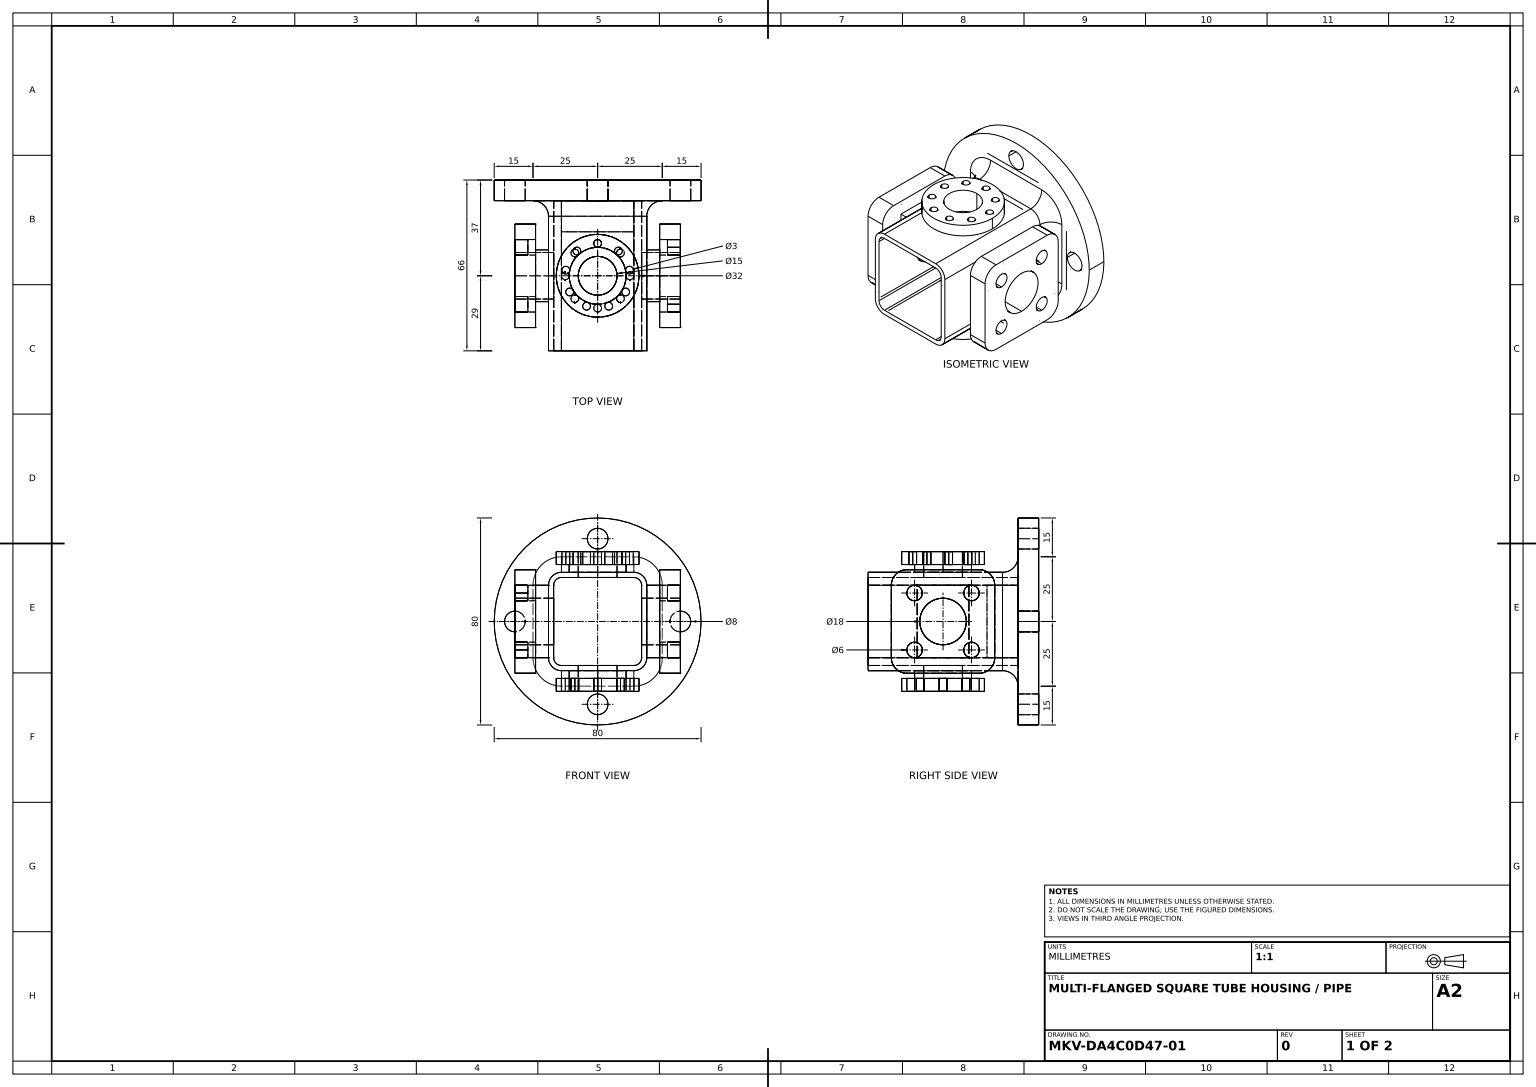
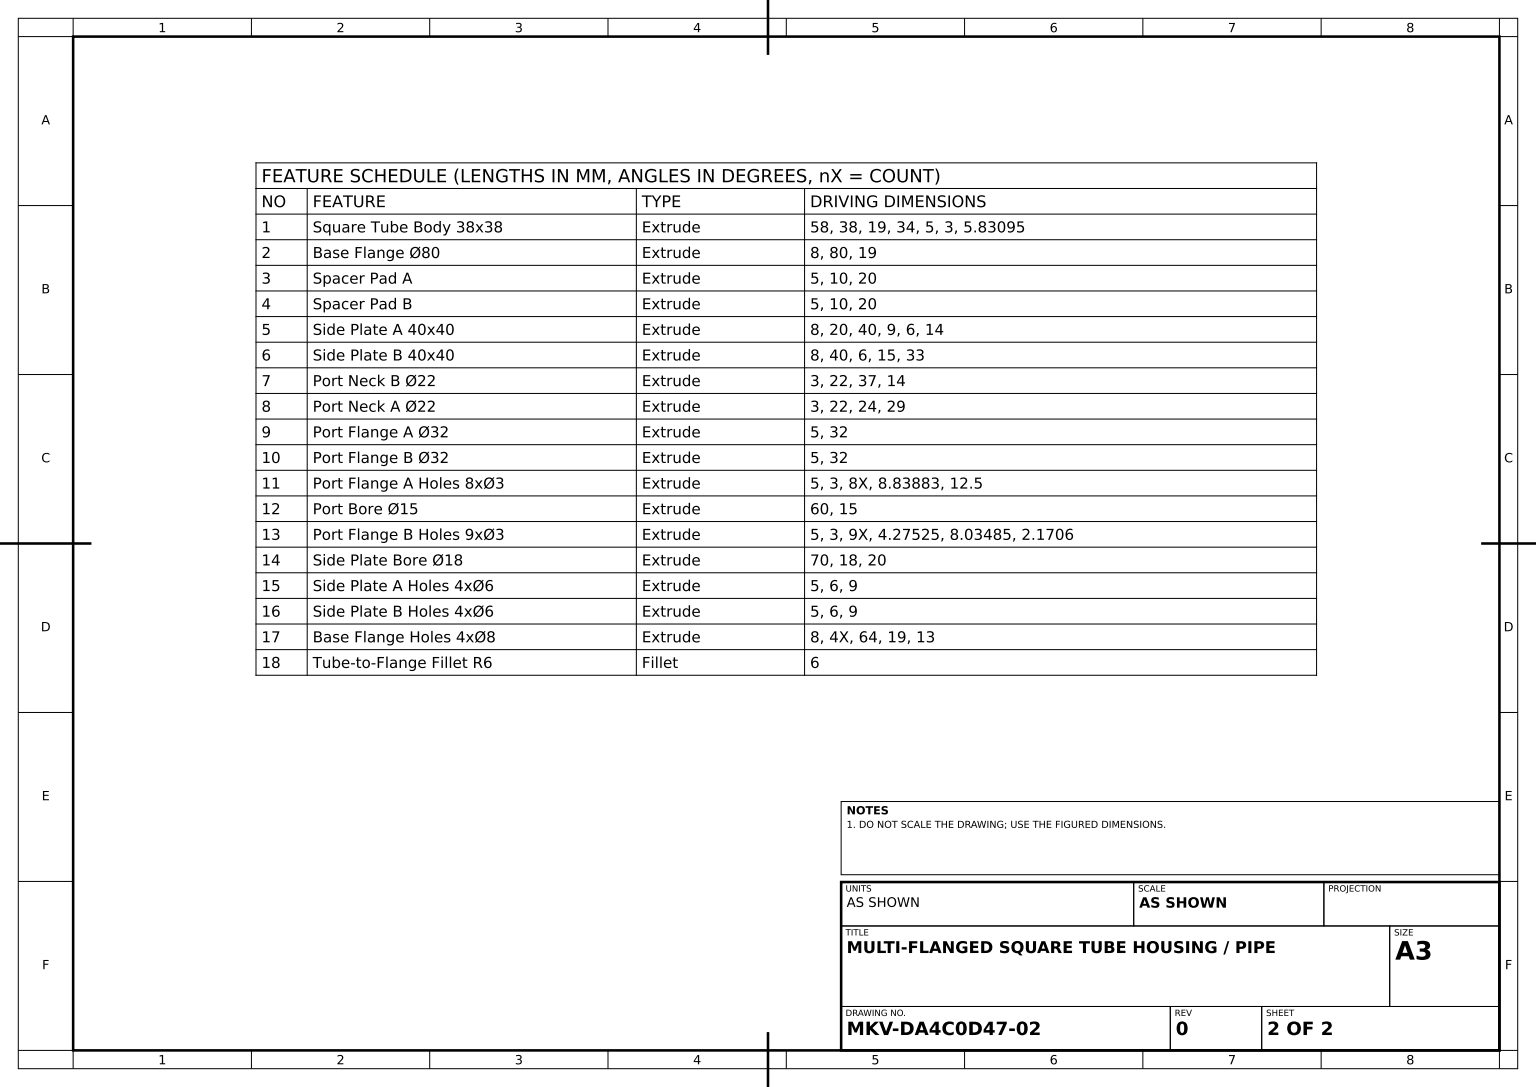
from build123d import *

# Parameters (mm, degrees)
SQUARE_TUBE_BODY_38X38_DEPTH   = 58
BASE_FLANGE_SKETCH_R           = 40
BASE_FLANGE_80_DEPTH           = 8
SPACER_PAD_A_DEPTH             = 5
SPACER_PAD_B_DEPTH             = 5
SIDE_PLATE_A_40X40_DEPTH       = 8
SIDE_START                     = 8
SIDE_PLATE_B_40X40_DEPTH       = 8
PORT_NECK_B_SKETCH_R           = 11
PORT_NECK_B_22_DEPTH           = 3
PORT_START                     = 3
PORT_NECK_A_SKETCH_R           = 11
PORT_NECK_A_22_DEPTH           = 3
PORT_FLANGE_A_SKETCH_R         = 16
PORT_FLANGE_A_32_DEPTH         = 5
PORT_START_2                   = 5
PORT_FLANGE_B_SKETCH_R         = 16
PORT_FLANGE_B_32_DEPTH         = 5
PORT_FLANGE_A_HOLES_SKETCH_R   = 1.5
PORT_FLANGE_A_HOLES_8X_3_DEPTH = 5
PORT_BORE_SKETCH_R             = 7.5
PORT_BORE_15_DEPTH             = 60
PORT_START_3                   = -5
PORT_FLANGE_B_HOLES_SKETCH_R   = 1.5
PORT_FLANGE_B_HOLES_9X_3_DEPTH = 5
SIDE_PLATE_BORE_SKETCH_R       = 9
SIDE_PLATE_BORE_18_DEPTH       = 70
SIDE_PLATE_A_HOLES_SKETCH_R    = 3
SIDE_PLATE_A_HOLES_4X_6_DEPTH  = 5
SIDE_START_2                   = -5
SIDE_PLATE_B_HOLES_SKETCH_R    = 3
SIDE_PLATE_B_HOLES_4X_6_DEPTH  = 5
BASE_FLANGE_HOLES_SKETCH_R     = 4
BASE_FLANGE_HOLES_4X_8_DEPTH   = 8
TUBE_TO_FLANGE_FILLET_R6_R     = 6


with BuildPart() as part:
    # Square Tube Profile Sketch → Square Tube Body 38x38 (new body)
    with BuildSketch(Plane.XY):
        with BuildLine():
            Line((5, 0), (33, 0))
            ThreePointArc((33, 0), (36.535533906, -1.464466094), (38, -5))
            Line((38, -5), (38, -33))
            ThreePointArc((38, -33), (36.535533906, -36.535533906), (33, -38))
            Line((33, -38), (5, -38))
            ThreePointArc((5, -38), (1.464466094, -36.535533906), (0, -33))
            Line((0, -33), (0, -5))
            ThreePointArc((0, -5), (1.464466094, -1.464466094), (5, 0))
        make_face()
        with BuildLine():
            Line((5, -2), (33, -2))
            ThreePointArc((33, -2), (35.121320344, -2.878679656), (36, -5))
            Line((36, -5), (36, -33))
            ThreePointArc((36, -33), (35.121320344, -35.121320344), (33, -36))
            Line((33, -36), (5, -36))
            ThreePointArc((5, -36), (2.878679656, -35.121320344), (2, -33))
            Line((2, -33), (2, -5))
            ThreePointArc((2, -5), (2.878679656, -2.878679656), (5, -2))
        make_face(mode=Mode.SUBTRACT)
    extrude(amount=SQUARE_TUBE_BODY_38X38_DEPTH)

    # Base Flange Sketch → Base Flange Ø80 (add)
    with BuildSketch(Plane(origin=(0, 0, 0), x_dir=(-1, 0, 0), z_dir=(0, 0, -1))):
        with Locations((-19, -19)):
            Circle(BASE_FLANGE_SKETCH_R)
    extrude(amount=BASE_FLANGE_80_DEPTH)

    # Spacer Pad A Sketch → Spacer Pad A (add)
    with BuildSketch(Plane(origin=(38, 0, 0), x_dir=(0, 0, -1), z_dir=(1, 0, 0))):
        Polygon((-19, -5), (-29, -5), (-39, -5), (-39, -33), (-19, -33), align=None)
    extrude(amount=SPACER_PAD_A_DEPTH)

    # Spacer Pad B Sketch → Spacer Pad B (add)
    with BuildSketch(Plane.ZY):
        Polygon((29, -5), (39, -5), (39, -33), (19, -33), (19, -5), align=None)
    extrude(amount=SPACER_PAD_B_DEPTH)

    # Side Plate A Sketch → Side Plate A 40x40 (add)
    with BuildSketch(Plane(origin=(43, 0, 0), x_dir=(0, 0, -1), z_dir=(1, 0, 0))):
        with BuildLine():
            Line((-9, -19), (-9, -5))
            ThreePointArc((-9, -5), (-10.757359313, -0.757359313), (-15, 1))
            Line((-15, 1), (-43, 1))
            ThreePointArc((-43, 1), (-47.242640687, -0.757359313), (-49, -5))
            Line((-49, -5), (-49, -33))
            ThreePointArc((-49, -33), (-47.242640687, -37.242640687), (-43, -39))
            Line((-43, -39), (-15, -39))
            ThreePointArc((-15, -39), (-10.757359313, -37.242640687), (-9, -33))
            Line((-9, -33), (-9, -19))
        make_face()
    extrude(amount=SIDE_PLATE_A_40X40_DEPTH)

    # Side Plate B Sketch → Side Plate B 40x40 (add)
    with BuildSketch(Plane.ZY.offset(5).offset(SIDE_START)):
        with BuildLine():
            Line((9, -5), (9, -33))
            ThreePointArc((9, -33), (10.757359313, -37.242640687), (15, -39))
            Line((15, -39), (43, -39))
            ThreePointArc((43, -39), (47.242640687, -37.242640687), (49, -33))
            Line((49, -33), (49, -5))
            ThreePointArc((49, -5), (47.242640687, -0.757359313), (43, 1))
            Line((43, 1), (15, 1))
            ThreePointArc((15, 1), (10.757359313, -0.757359313), (9, -5))
        make_face()
    extrude(amount=-SIDE_PLATE_B_40X40_DEPTH)

    # Port Neck B Sketch → Port Neck B Ø22 (add)
    with BuildSketch(Plane(origin=(0, 0, 0), x_dir=(1, 0, 0), z_dir=(0, 1, 0))):
        with Locations((19, -29)):
            Circle(PORT_NECK_B_SKETCH_R)
    extrude(amount=PORT_NECK_B_22_DEPTH)

    # Port Neck A Sketch → Port Neck A Ø22 (add)
    with BuildSketch(Plane.XZ.offset(38).offset(PORT_START)):
        with Locations((19, 29)):
            Circle(PORT_NECK_A_SKETCH_R)
    extrude(amount=-PORT_NECK_A_22_DEPTH)

    # Port Flange A Sketch → Port Flange A Ø32 (add)
    with BuildSketch(Plane.XZ.offset(41)):
        with Locations(Location((19, 29, 0), (0, 0, 270))):
            Circle(PORT_FLANGE_A_SKETCH_R)
    extrude(amount=PORT_FLANGE_A_32_DEPTH)

    # Port Flange B Sketch → Port Flange B Ø32 (add)
    with BuildSketch(Plane(origin=(0, 3, 0), x_dir=(1, 0, 0), z_dir=(0, 1, 0)).offset(PORT_START_2)):
        with Locations(Location((19, -29, 0), (0, 0, 90))):
            Circle(PORT_FLANGE_B_SKETCH_R)
    extrude(amount=-PORT_FLANGE_B_32_DEPTH)

    # Port Flange A Holes Sketch → Port Flange A Holes 8xØ3 (cut)
    with BuildSketch(Plane.XZ.offset(46)):
        with Locations(Location((31.5, 29, 0), (0, 0, 270))):
            Circle(PORT_FLANGE_A_HOLES_SKETCH_R)
        with Locations(Location((27.838834765, 20.161165235, 0), (0, 0, 270))):
            Circle(PORT_FLANGE_A_HOLES_SKETCH_R)
        with Locations(Location((19, 16.5, 0), (0, 0, 270))):
            Circle(PORT_FLANGE_A_HOLES_SKETCH_R)
        with Locations(Location((10.161165235, 20.161165235, 0), (0, 0, 270))):
            Circle(PORT_FLANGE_A_HOLES_SKETCH_R)
        with Locations(Location((6.5, 29, 0), (0, 0, 270))):
            Circle(PORT_FLANGE_A_HOLES_SKETCH_R)
        with Locations(Location((10.161165235, 37.838834765, 0), (0, 0, 270))):
            Circle(PORT_FLANGE_A_HOLES_SKETCH_R)
        with Locations(Location((19, 41.5, 0), (0, 0, 270))):
            Circle(PORT_FLANGE_A_HOLES_SKETCH_R)
        with Locations(Location((27.838834765, 37.838834765, 0), (0, 0, 270))):
            Circle(PORT_FLANGE_A_HOLES_SKETCH_R)
    extrude(amount=-PORT_FLANGE_A_HOLES_8X_3_DEPTH, mode=Mode.SUBTRACT)

    # Port Bore Sketch → Port Bore Ø15 (cut)
    with BuildSketch(Plane.XZ.offset(46)):
        with Locations(Location((19, 29, 0), (0, 0, 270))):
            Circle(PORT_BORE_SKETCH_R)
    extrude(amount=-PORT_BORE_15_DEPTH, mode=Mode.SUBTRACT)

    # Port Flange B Holes Sketch → Port Flange B Holes 9xØ3 (cut)
    with BuildSketch(Plane(origin=(0, 8, 0), x_dir=(1, 0, 0), z_dir=(0, 1, 0)).offset(PORT_START_3)):
        with Locations(Location((19, -16.5, 0), (0, 0, 90))):
            Circle(PORT_FLANGE_B_HOLES_SKETCH_R)
        with Locations(Location((27.034845121, -19.424444461, 0), (0, 0, 180))):
            Circle(PORT_FLANGE_B_HOLES_SKETCH_R)
        with Locations(Location((31.310096913, -26.829397779, 0), (0, 0, 180))):
            Circle(PORT_FLANGE_B_HOLES_SKETCH_R)
        with Locations(Location((29.825317547, -35.25, 0), (0, 0, 180))):
            Circle(PORT_FLANGE_B_HOLES_SKETCH_R)
        with Locations(Location((23.275251792, -40.74615776, 0), (0, 0, 180))):
            Circle(PORT_FLANGE_B_HOLES_SKETCH_R)
        with Locations(Location((14.724748208, -40.74615776, 0), (0, 0, 180))):
            Circle(PORT_FLANGE_B_HOLES_SKETCH_R)
        with Locations(Location((8.174682453, -35.25, 0), (0, 0, 180))):
            Circle(PORT_FLANGE_B_HOLES_SKETCH_R)
        with Locations(Location((6.689903087, -26.829397779, 0), (0, 0, 180))):
            Circle(PORT_FLANGE_B_HOLES_SKETCH_R)
        with Locations(Location((10.965154879, -19.424444461, 0), (0, 0, 180))):
            Circle(PORT_FLANGE_B_HOLES_SKETCH_R)
    extrude(amount=PORT_FLANGE_B_HOLES_9X_3_DEPTH, mode=Mode.SUBTRACT)

    # Side Plate Bore Sketch → Side Plate Bore Ø18 (cut)
    with BuildSketch(Plane(origin=(51, 0, 0), x_dir=(0, 0, -1), z_dir=(1, 0, 0))):
        with Locations((-29, -19)):
            Circle(SIDE_PLATE_BORE_SKETCH_R)
    extrude(amount=-SIDE_PLATE_BORE_18_DEPTH, mode=Mode.SUBTRACT)

    # Side Plate A Holes Sketch → Side Plate A Holes 4xØ6 (cut)
    with BuildSketch(Plane(origin=(51, 0, 0), x_dir=(0, 0, -1), z_dir=(1, 0, 0))):
        with Locations(Location((-18, -8, 0), (0, 0, 90))):
            Circle(SIDE_PLATE_A_HOLES_SKETCH_R)
        with Locations(Location((-40, -30, 0), (0, 0, 90))):
            Circle(SIDE_PLATE_A_HOLES_SKETCH_R)
        with Locations(Location((-18, -30, 0), (0, 0, 90))):
            Circle(SIDE_PLATE_A_HOLES_SKETCH_R)
        with Locations(Location((-40, -8, 0), (0, 0, 90))):
            Circle(SIDE_PLATE_A_HOLES_SKETCH_R)
    extrude(amount=-SIDE_PLATE_A_HOLES_4X_6_DEPTH, mode=Mode.SUBTRACT)

    # Side Plate B Holes Sketch → Side Plate B Holes 4xØ6 (cut)
    with BuildSketch(Plane.ZY.offset(13).offset(SIDE_START_2)):
        with Locations(Location((18, -8, 0), (0, 0, 90))):
            Circle(SIDE_PLATE_B_HOLES_SKETCH_R)
        with Locations(Location((40, -8, 0), (0, 0, 90))):
            Circle(SIDE_PLATE_B_HOLES_SKETCH_R)
        with Locations(Location((40, -30, 0), (0, 0, 90))):
            Circle(SIDE_PLATE_B_HOLES_SKETCH_R)
        with Locations(Location((18, -30, 0), (0, 0, 90))):
            Circle(SIDE_PLATE_B_HOLES_SKETCH_R)
    extrude(amount=SIDE_PLATE_B_HOLES_4X_6_DEPTH, mode=Mode.SUBTRACT)

    # Base Flange Holes Sketch → Base Flange Holes 4xØ8 (cut)
    with BuildSketch(Plane(origin=(0, 0, -8), x_dir=(-1, 0, 0), z_dir=(0, 0, -1))):
        with Locations((-19, 13)):
            Circle(BASE_FLANGE_HOLES_SKETCH_R)
        with Locations((13, -19)):
            Circle(BASE_FLANGE_HOLES_SKETCH_R)
        with Locations((-19, -51)):
            Circle(BASE_FLANGE_HOLES_SKETCH_R)
        with Locations((-51, -19)):
            Circle(BASE_FLANGE_HOLES_SKETCH_R)
    extrude(amount=-BASE_FLANGE_HOLES_4X_8_DEPTH, mode=Mode.SUBTRACT)

    # Tube-to-Flange Fillet R6
    tube_to_flange_fillet_r6_edges = [part.edges().sort_by_distance(p)[0] for p in [
        (19, -38, 0),
        (1.464466094, -36.535533906, 0),
        (0, -19, 0),
        (1.464466094, -1.464466094, 0),
        (19, 0, 0),
        (36.535533906, -1.464466094, 0),
        (38, -19, 0),
        (36.535533906, -36.535533906, 0),
    ]]
    fillet(tube_to_flange_fillet_r6_edges, radius=TUBE_TO_FLANGE_FILLET_R6_R)


solid = part.part
